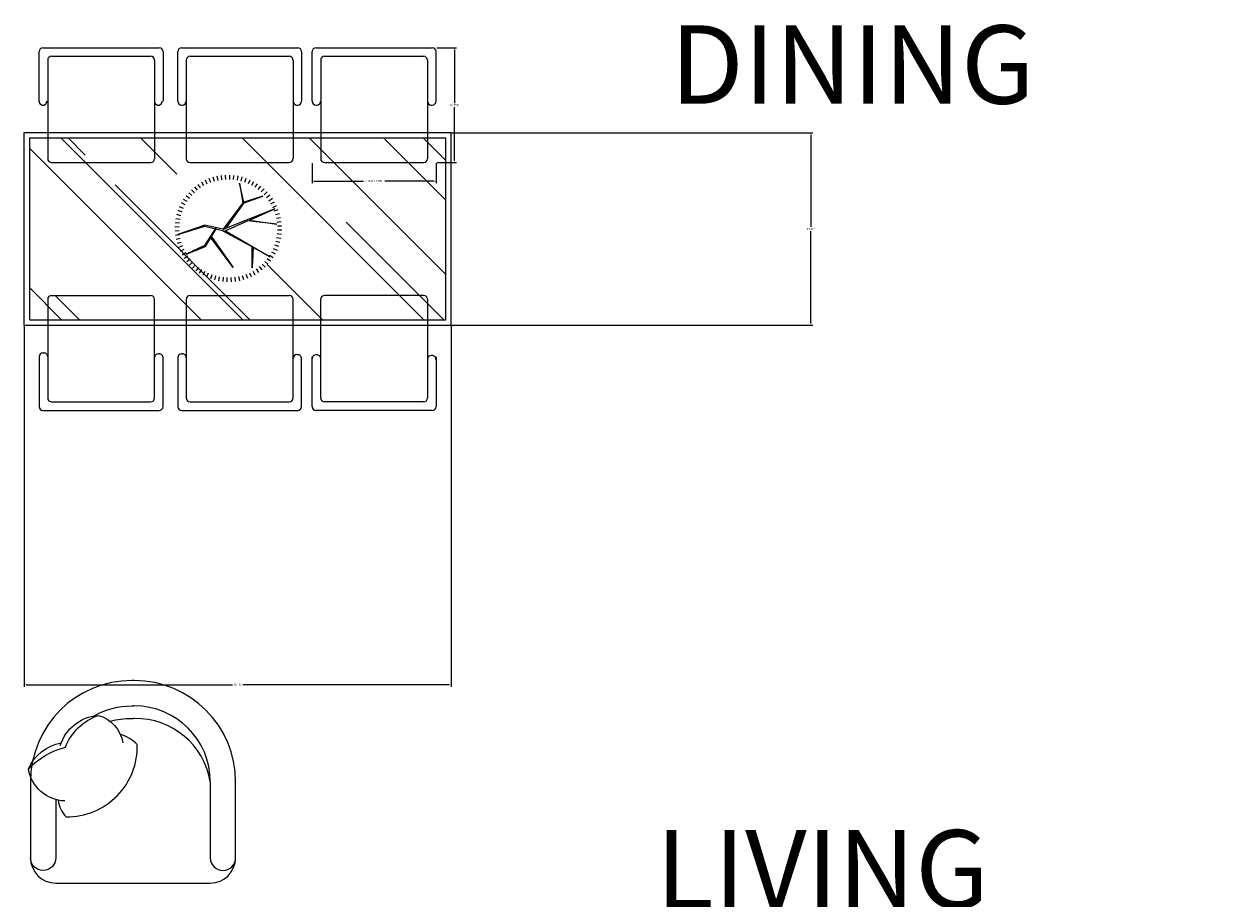
# Model space of a CAD drawing. Units: inches. Extents: x 1676 to 2199, y 1657 to 2783.
# Tile 4 of 10: x 1788 to 1895, y 1985 to 2063. Entities that reach past the tile are written whole.
import ezdxf

# ---------------------------------------------------------------- set-up
doc = ezdxf.new("R2010")
doc.units = ezdxf.units.IN
for name, color, linetype, lineweight in [('A-ANNO-DIMS', 2, 'Continuous', 18), ('A-AREA-IDEN', 7, 'Continuous', 18), ('A-FURN', 8, 'Continuous', 13), ('A-FURN-PATT', 8, 'Continuous', 13)]:
    doc.layers.add(name, color=color, linetype=linetype, lineweight=lineweight)
doc.styles.get("Standard").update_dxf_attribs({"font": 'arial.ttf'})
doc.dimstyles.get("Standard").update_dxf_attribs({"dimtxt": 0.18, "dimasz": 0.18, "dimexe": 0.18, "dimexo": 0.0625, "dimgap": 0.09, "dimtad": 0, "dimtih": 1, "dimtoh": 1, "dimdec": 4, "dimzin": 0, "dimdsep": 46, "dimtxsty": 'Standard', "dimcen": 0.09, "dimadec": 0, "dimazin": 0, "dimtfac": 1, "dimtdec": 4, "dimtofl": 0, "dimtmove": 0, "dimatfit": 3, "dimfxl": 1, "dimtolj": 1, "dimtzin": 0, "dimarcsym": 0})

# ---------------------------------------------------------------- blocks, each defined once
blk = doc.blocks.new('CHAIR-DINING')
for p, q in [((-1.11, 5.48), (-1.11, 9.92)), ((-0.76, 10.27), (9.62, 10.27)), ((9.96, 9.92), (9.96, 5.48)), ((-0.34, 9.16), (-0.34, 0.34)), ((0, 9.5), (8.85, 9.5)), ((9.2, 9.16), (9.2, 0.34)), ((-0.76, 5.13), (-0.69, 5.13)), ((9.54, 5.13), (9.62, 5.13)), ((0, 0), (8.85, 0))]:
    blk.add_line(p, q)
for centre, start, end in [((-0.76, 9.92), 90, 180), ((9.62, 9.92), 0, 90), ((0, 9.16), 90, 180), ((8.85, 9.16), 0, 90), ((-0.76, 5.48), 180, 270), ((-0.69, 5.48), 270, 0), ((9.54, 5.48), 180, 270), ((9.62, 5.48), 270, 0), ((0, 0.34), 180, 270), ((8.85, 0.34), 270, 0)]:
    blk.add_arc(centre, 0.343, start, end)
blk = doc.blocks.new('*D17')
at = {"layer": 'A-ANNO-DIMS', "color": 0, "lineweight": -2, "transparency": 16777216}
for p, q in [((1813.71, 2050.79), (1813.71, 2049.02)), ((1824.78, 2050.79), (1824.78, 2049.02)), ((1813.89, 2049.2), (1818.29, 2049.2)), ((1824.6, 2049.2), (1820.2, 2049.2))]:
    blk.add_line(p, q, dxfattribs=at)
at = {"layer": 'A-ANNO-DIMS', "color": 0, "transparency": 16777216}
for points in [[(1813.89, 2049.23), (1813.89, 2049.17), (1813.71, 2049.2)], [(1824.6, 2049.23), (1824.6, 2049.17), (1824.78, 2049.2)]]:
    blk.add_solid(points, dxfattribs=at)
at = {"layer": 'Defpoints', "color": 0, "transparency": 16777216}
for p in [(1813.71, 2050.86), (1824.78, 2050.86), (1824.78, 2049.2)]:
    blk.add_point(p, dxfattribs=at)
at = {"layer": 'A-ANNO-DIMS', "color": 0, "transparency": 16777216, "insert": (1819.25, 2049.2), "char_height": 0.18, "attachment_point": 5}
blk.add_mtext('\\A1;CHAIR 11 TYP.', dxfattribs=at)
blk = doc.blocks.new('*D18')
at = {"layer": 'A-ANNO-DIMS', "color": 0, "lineweight": -2, "transparency": 16777216}
for p, q in [((1824.84, 2061.12), (1826.62, 2061.12)), ((1826.44, 2060.94), (1826.44, 2056.17)), ((1826.44, 2051.04), (1826.44, 2055.81)), ((1824.84, 2050.86), (1826.62, 2050.86))]:
    blk.add_line(p, q, dxfattribs=at)
at = {"layer": 'A-ANNO-DIMS', "color": 0, "transparency": 16777216}
for points in [[(1826.41, 2060.94), (1826.47, 2060.94), (1826.44, 2061.12)], [(1826.41, 2051.04), (1826.47, 2051.04), (1826.44, 2050.86)]]:
    blk.add_solid(points, dxfattribs=at)
at = {"layer": 'Defpoints', "color": 0, "transparency": 16777216}
for p in [(1824.78, 2061.12), (1826.44, 2061.12), (1824.78, 2050.86)]:
    blk.add_point(p, dxfattribs=at)
at = {"layer": 'A-ANNO-DIMS', "color": 0, "transparency": 16777216, "insert": (1826.44, 2055.99), "char_height": 0.18, "attachment_point": 5}
blk.add_mtext('\\A1;10 TYP.', dxfattribs=at)
blk = doc.blocks.new('*D54')
at = {"layer": 'A-ANNO-DIMS', "color": 0, "lineweight": -2, "transparency": 16777216}
for p, q in [((1787.97, 2036.27), (1787.97, 2004)), ((1826.13, 2036.27), (1826.13, 2004)), ((1788.15, 2004.18), (1806.59, 2004.18)), ((1825.95, 2004.18), (1807.51, 2004.18))]:
    blk.add_line(p, q, dxfattribs=at)
at = {"layer": 'A-ANNO-DIMS', "color": 0, "transparency": 16777216}
for points in [[(1788.15, 2004.21), (1788.15, 2004.15), (1787.97, 2004.18)], [(1825.95, 2004.21), (1825.95, 2004.15), (1826.13, 2004.18)]]:
    blk.add_solid(points, dxfattribs=at)
at = {"layer": 'Defpoints', "color": 0, "transparency": 16777216}
for p in [(1787.97, 2036.33), (1826.13, 2036.33), (1787.97, 2004.18)]:
    blk.add_point(p, dxfattribs=at)
at = {"layer": 'A-ANNO-DIMS', "color": 0, "transparency": 16777216, "insert": (1807.05, 2004.18), "char_height": 0.18, "attachment_point": 5}
blk.add_mtext('\\A1;38.164', dxfattribs=at)
blk = doc.blocks.new('*D55')
at = {"layer": 'A-ANNO-DIMS', "color": 0, "lineweight": -2, "transparency": 16777216}
for p, q in [((1826.2, 2053.5), (1858.46, 2053.5)), ((1858.28, 2053.32), (1858.28, 2045.1)), ((1858.28, 2036.51), (1858.28, 2044.74)), ((1826.2, 2036.33), (1858.46, 2036.33))]:
    blk.add_line(p, q, dxfattribs=at)
at = {"layer": 'A-ANNO-DIMS', "color": 0, "transparency": 16777216}
for points in [[(1858.25, 2053.32), (1858.31, 2053.32), (1858.28, 2053.5)], [(1858.25, 2036.51), (1858.31, 2036.51), (1858.28, 2036.33)]]:
    blk.add_solid(points, dxfattribs=at)
at = {"layer": 'Defpoints', "color": 0, "transparency": 16777216}
for p in [(1826.13, 2053.5), (1826.13, 2036.33), (1858.28, 2036.33)]:
    blk.add_point(p, dxfattribs=at)
at = {"layer": 'A-ANNO-DIMS', "color": 0, "transparency": 16777216, "insert": (1858.28, 2044.92), "char_height": 0.18, "attachment_point": 5}
blk.add_mtext('\\A1;17.174', dxfattribs=at)

msp = doc.modelspace()

# ---------------------------------------------------------------- hatches: boundary and pattern name
at = {"layer": 'A-FURN-PATT'}
h = msp.add_hatch(dxfattribs=at)
h.set_pattern_fill('AR-RROOF', color=256, scale=11.449163, angle=-45, style=0)
h.set_pattern_definition([(315, (2164.764, 3007.215), (25.9065, -9.71494), [171.7375, -22.8983, 57.2458, -11.4492]), (315, (2179.579, 3000.495), (2.6716, 18.86317), [34.3475, -3.7782, 68.695, -8.5869]), (315, (2175.693, 3010.048), (47.522235, -36.67389), [91.5933, -16.02883, 45.79665, -11.44916])])
h.paths.add_polyline_path([(1788.4461, 2036.8061), (1825.6559, 2036.8061), (1825.6559, 2053.0257), (1788.4461, 2053.0257)])

# ---------------------------------------------------------------- linework, layer by layer
at = {"layer": 'A-FURN'}
for p, q in [((1789.3226, 2056.3323), (1789.3226, 2060.7787)), ((1789.666, 2061.1221), (1800.0466, 2061.1221)), ((1800.3901, 2060.7787), (1800.3901, 2056.3323)), ((1790.0858, 2060.0154), (1790.0858, 2051.199)), ((1790.4293, 2060.3589), (1799.2833, 2060.3589)), ((1799.6268, 2060.0154), (1799.6268, 2051.199)), ((1789.666, 2055.9888), (1789.7424, 2055.9888)), ((1799.9703, 2055.9888), (1800.0466, 2055.9888)), ((1826.1329, 2053.5028), (1787.969, 2053.5028)), ((1787.969, 2053.5028), (1787.969, 2036.329)), ((1826.1329, 2036.329), (1826.1329, 2053.5028)), ((1825.6559, 2053.0257), (1788.4461, 2053.0257)), ((1788.4461, 2053.0257), (1788.4461, 2036.8061)), ((1825.6559, 2036.8061), (1825.6559, 2053.0257)), ((1790.4293, 2050.8555), (1799.2833, 2050.8555)), ((1803.743, 2048.5876), (1803.5272, 2048.9023)), ((1804.0346, 2048.7712), (1803.8442, 2049.1019)), ((1804.3398, 2048.9313), (1804.1759, 2049.2759)), ((1804.6566, 2049.067), (1804.5202, 2049.4234)), ((1804.983, 2049.1774), (1804.875, 2049.5434)), ((1805.3171, 2049.2618), (1805.2382, 2049.6352)), ((1805.6568, 2049.3198), (1805.6074, 2049.6983)), ((1806, 2049.351), (1805.9804, 2049.7321)), ((1806.3446, 2049.3551), (1806.355, 2049.7366)), ((1806.6884, 2049.3322), (1806.7287, 2049.7117)), ((1807.0294, 2049.2824), (1807.0994, 2049.6576)), ((1807.2248, 2049.0272), (1807.5315, 2047.2539)), ((1807.5997, 2047.3221), (1807.2248, 2049.0272)), ((1807.3655, 2049.206), (1807.4646, 2049.5745)), ((1807.6945, 2049.1034), (1807.8222, 2049.463)), ((1808.0144, 2048.9754), (1808.17, 2049.3239)), ((1808.3233, 2048.8226), (1808.5058, 2049.1578)), ((1808.6193, 2048.6461), (1808.8275, 2048.9659)), ((1802.7459, 2047.6435), (1802.4434, 2047.8761)), ((1802.9666, 2047.9082), (1802.6832, 2048.1638)), ((1803.2073, 2048.1548), (1802.9449, 2048.4319)), ((1803.4667, 2048.3817), (1803.2268, 2048.6785)), ((1809.3036, 2047.8677), (1807.5997, 2047.3221)), ((1807.6337, 2047.2539), (1809.3036, 2047.8677)), ((1808.9005, 2048.4469), (1809.1331, 2048.7494)), ((1809.1652, 2048.2263), (1809.4209, 2048.5096)), ((1809.4118, 2047.9855), (1809.6889, 2048.2479)), ((1809.6387, 2047.7262), (1809.9356, 2047.966)), ((1802.2175, 2046.7574), (1801.869, 2046.913)), ((1802.3702, 2047.0663), (1802.035, 2047.2488)), ((1802.5467, 2047.3623), (1802.2269, 2047.5705)), ((1807.5315, 2047.2539), (1805.7253, 2044.8668)), ((1810.3941, 2046.7083), (1805.7253, 2044.8668)), ((1805.9639, 2044.9009), (1807.6337, 2047.2539)), ((1808.1204, 2045.7183), (1810.3941, 2046.7083)), ((1809.8446, 2047.4498), (1810.1593, 2047.6657)), ((1810.0282, 2047.1582), (1810.3589, 2047.3487)), ((1810.1883, 2046.853), (1810.5329, 2047.017)), ((1801.9104, 2045.7724), (1801.5353, 2045.8424)), ((1801.9869, 2046.1084), (1801.6183, 2046.2076)), ((1802.0894, 2046.4374), (1801.7298, 2046.5652)), ((1805.9298, 2044.7645), (1807.9425, 2045.6409)), ((1810.5645, 2045.3443), (1807.9425, 2045.6409)), ((1808.1204, 2045.7183), (1810.5645, 2045.3443)), ((1810.324, 2046.5363), (1810.6804, 2046.6726)), ((1810.4344, 2046.2098), (1810.8004, 2046.3178)), ((1810.5189, 2045.8757), (1810.8922, 2045.9547)), ((1801.8377, 2045.0876), (1801.4562, 2045.098)), ((1801.8418, 2044.743), (1801.4607, 2044.7234)), ((1801.8606, 2045.4314), (1801.4811, 2045.4717)), ((1804.1237, 2045.2761), (1801.7041, 2044.4235)), ((1801.7041, 2044.4235), (1804.1237, 2045.1738)), ((1805.1119, 2045.0374), (1804.0896, 2043.4346)), ((1805.7253, 2044.9009), (1804.1237, 2045.2761)), ((1804.1237, 2045.1738), (1805.9298, 2044.7304)), ((1804.1918, 2043.3664), (1805.146, 2044.935)), ((1808.3494, 2043.3187), (1805.7594, 2044.7304)), ((1805.9639, 2044.7645), (1809.9511, 2042.4457)), ((1810.5768, 2045.536), (1810.9553, 2045.5854)), ((1810.608, 2045.1928), (1810.9891, 2045.2124)), ((1810.6121, 2044.8482), (1810.9936, 2044.8378)), ((1801.873, 2044.3998), (1801.4946, 2044.3504)), ((1801.931, 2044.0601), (1801.5576, 2043.9812)), ((1802.0155, 2043.726), (1801.6494, 2043.618)), ((1806.6455, 2041.4908), (1804.6348, 2044.1848)), ((1804.7371, 2044.1848), (1806.6455, 2041.4908)), ((1810.3604, 2043.4984), (1810.72, 2043.3706)), ((1810.463, 2043.8274), (1810.8315, 2043.7282)), ((1810.5394, 2044.1634), (1810.9146, 2044.0935)), ((1810.5892, 2044.5044), (1810.9687, 2044.4641)), ((1802.1259, 2043.3996), (1801.7694, 2043.2632)), ((1802.2616, 2043.0828), (1801.9169, 2042.9189)), ((1802.4217, 2042.7776), (1802.091, 2042.5872)), ((1802.6053, 2042.486), (1802.2905, 2042.2702)), ((1804.0896, 2043.4346), (1802.4538, 2042.6844)), ((1802.4538, 2042.6844), (1804.1918, 2043.3664)), ((1808.3494, 2041.4567), (1808.3494, 2043.3187)), ((1808.4295, 2043.275), (1808.3494, 2041.4567)), ((1809.9511, 2042.4457), (1808.4295, 2043.275)), ((1809.9031, 2042.5736), (1810.223, 2042.3654)), ((1810.0796, 2042.8695), (1810.4148, 2042.6871)), ((1810.2324, 2043.1784), (1810.5809, 2043.0228)), ((1802.8111, 2042.2096), (1802.5143, 2041.9698)), ((1803.0381, 2041.9503), (1802.761, 2041.6879)), ((1803.2847, 2041.7096), (1803.029, 2041.4262)), ((1803.5494, 2041.4889), (1803.3167, 2041.1864)), ((1808.7069, 2041.3482), (1808.9227, 2041.0335)), ((1808.9832, 2041.5541), (1809.223, 2041.2573)), ((1809.2425, 2041.7811), (1809.5049, 2041.5039)), ((1809.4833, 2042.0276), (1809.7666, 2041.772)), ((1809.7039, 2042.2924), (1810.0064, 2042.0597)), ((1803.8306, 2041.2897), (1803.6224, 2040.9699)), ((1804.1265, 2041.1132), (1803.9441, 2040.778)), ((1804.4355, 2040.9604), (1804.2798, 2040.612)), ((1804.7554, 2040.8324), (1804.6276, 2040.4728)), ((1805.0844, 2040.7299), (1804.9852, 2040.3613)), ((1805.4204, 2040.6534), (1805.3505, 2040.2783)), ((1805.7614, 2040.6036), (1805.7211, 2040.2241)), ((1806.1053, 2040.5807), (1806.0949, 2040.1992)), ((1806.4498, 2040.5848), (1806.4694, 2040.2037)), ((1806.793, 2040.616), (1806.8424, 2040.2376)), ((1807.1327, 2040.674), (1807.2117, 2040.3006)), ((1807.4668, 2040.7584), (1807.5748, 2040.3924)), ((1807.7933, 2040.8689), (1807.9297, 2040.5124)), ((1808.1101, 2041.0045), (1808.274, 2040.6599)), ((1808.4152, 2041.1647), (1808.6057, 2040.834)), ((1790.0858, 2038.6328), (1790.0858, 2029.8164)), ((1790.4293, 2038.9762), (1799.2833, 2038.9762)), ((1799.6268, 2029.8164), (1799.6268, 2038.6328)), ((1802.465, 2038.6328), (1802.465, 2029.8164)), ((1802.8084, 2038.9762), (1811.6625, 2038.9762)), ((1812.0059, 2029.8164), (1812.0059, 2038.6328)), ((1814.4751, 2029.8164), (1814.4751, 2038.6328)), ((1823.6726, 2038.9762), (1814.8186, 2038.9762)), ((1824.0161, 2038.6328), (1824.0161, 2029.8164)), ((1787.969, 2036.329), (1826.1329, 2036.329)), ((1788.4461, 2036.8061), (1825.6559, 2036.8061)), ((1789.6683, 2033.8406), (1789.7446, 2033.8401)), ((1789.3226, 2033.4995), (1789.3226, 2029.0531)), ((1799.9723, 2033.7724), (1800.0487, 2033.7718)), ((1800.3901, 2029.0531), (1800.3901, 2033.4995)), ((1801.7017, 2033.4995), (1801.7017, 2029.0531)), ((1802.0472, 2033.7586), (1802.1235, 2033.7581)), ((1812.3512, 2033.6903), (1812.4275, 2033.6898)), ((1812.7692, 2029.0531), (1812.7692, 2033.4995)), ((1813.7118, 2029.0531), (1813.7118, 2033.4995)), ((1814.1334, 2033.6785), (1814.057, 2033.679)), ((1824.4374, 2033.6102), (1824.3611, 2033.6107)), ((1824.7794, 2033.4995), (1824.7794, 2029.0531)), ((1789.666, 2028.7096), (1800.0466, 2028.7096)), ((1790.4293, 2029.4729), (1799.2833, 2029.4729)), ((1802.0452, 2028.7096), (1812.4257, 2028.7096)), ((1802.8084, 2029.4729), (1811.6625, 2029.4729)), ((1824.4359, 2028.7096), (1814.0553, 2028.7096)), ((1823.6726, 2029.4729), (1814.8186, 2029.4729))]:
    msp.add_line(p, q, dxfattribs=at)
at = {"layer": 'A-FURN', "ltscale": 0.03}
msp.add_lwpolyline([(1797.7122, 1986.4536), (1804.6154, 1986.4536, 0.41421356), (1806.8787, 1988.7169), (1806.8787, 1995.5069, 0.41421356), (1797.8254, 2004.5603), (1797.7122, 2004.5603), (1797.5991, 2004.5603, 0.41421356), (1788.5457, 1995.5069), (1788.5457, 1988.7169, 0.41421356), (1790.8091, 1986.4536), (1797.7122, 1986.4536)], format="xyb", dxfattribs=at)
at = {"layer": 'A-FURN'}
for points in [[(1794.2286, 2001.4014, -0.13059149), (1797.5991, 2002.2969), (1797.7122, 2002.2969)], [(1804.6154, 1995.5069, 0.41421356), (1797.8254, 2002.2969), (1797.7122, 2002.2969)], [(1788.3606, 1996.6493, -0.14772988), (1791.6682, 1998.5942, -0.21334276), (1794.5866, 2001.4467, -0.17866181)], [(1791.2112, 1998.7492, -0.30666349), (1794.5866, 2001.4467, -0.30632997), (1796.7916, 1998.9832, 0.87284716)], [(1795.6696, 2000.9214, -0.07238424), (1797.5991, 2001.1653), (1797.7122, 2001.1653)], [(1804.6154, 1995.5069, 0.37271891), (1797.8254, 2001.1653), (1797.7122, 2001.1653)], [(1791.0329, 1993.8658, 0.16554063), (1791.733, 1992.3706, 0.42598917), (1798.0887, 1998.8535, 0.12152332), (1796.58, 1999.7471, -7.11546429)], [(1791.6033, 1993.7968, -0.35677236), (1788.3606, 1996.6493, -0.24954205), (1791.2988, 1999, 9.61688035)], [(1804.6154, 1995.5071), (1804.6154, 1988.7169, 0.41421356), (1805.7471, 1987.5853), (1805.7471, 1987.5853, 0.41421356), (1806.8787, 1988.7169)], [(1790.8091, 1993.9202), (1790.8091, 1988.7169, -0.41421356), (1789.6774, 1987.5853), (1789.6774, 1987.5853, -0.41421356), (1788.5457, 1988.7169)]]:
    msp.add_lwpolyline(points, format="xyb", dxfattribs=at)
for centre, start, end in [((1789.666, 2060.7787), 90, 180), ((1800.0466, 2060.7787), 0, 90), ((1790.4293, 2060.0154), 90, 180), ((1799.2833, 2060.0154), 0, 90), ((1789.666, 2056.3323), 180, 0.103974), ((1799.9703, 2056.3323), 180, 0.103974), ((1790.4293, 2051.199), 180, 270), ((1799.2833, 2051.199), 270, 0), ((1790.4293, 2038.6328), 90, 180), ((1799.2833, 2038.6328), 0, 90), ((1802.8084, 2038.6328), 90, 180), ((1811.6625, 2038.6328), 0, 90), ((1814.8186, 2038.6328), 90, 180), ((1823.6726, 2038.6328), 0, 90), ((1789.666, 2033.4972), 89.620247, 179.620246), ((1789.7424, 2033.4967), 359.620246, 89.620247), ((1799.9701, 2033.4289), 89.620247, 179.620246), ((1800.0464, 2033.4284), 359.620246, 89.620247), ((1802.0449, 2033.4151), 89.620247, 179.620246), ((1802.1212, 2033.4146), 359.620246, 89.620247), ((1812.3489, 2033.3468), 89.620247, 179.620246), ((1812.4252, 2033.3463), 359.620246, 89.620247), ((1814.0548, 2033.3355), 89.620247, 179.620246), ((1814.1311, 2033.335), 359.620246, 89.620247), ((1824.3588, 2033.2672), 89.620247, 179.620246), ((1824.4351, 2033.2667), 359.620246, 89.620247), ((1790.4293, 2029.8164), 180, 270), ((1799.2833, 2029.8164), 270, 0), ((1802.8084, 2029.8164), 180, 270), ((1811.6625, 2029.8164), 270, 0), ((1814.8186, 2029.8164), 180, 270), ((1823.6726, 2029.8164), 270, 0), ((1789.666, 2029.0531), 180, 270), ((1800.0466, 2029.0531), 270, 0), ((1802.0452, 2029.0531), 180, 270), ((1812.4257, 2029.0531), 270, 0), ((1814.0553, 2029.0531), 180, 270), ((1824.4359, 2029.0531), 270, 0)]:
    msp.add_arc(centre, 0.3435, start, end, dxfattribs=at)

# ---------------------------------------------------------------- block references
for p in [(1802.8084, 2050.8555), (1814.8186, 2050.8555)]:
    msp.add_blockref('CHAIR-DINING', p, dxfattribs=at)

# ---------------------------------------------------------------- texts
at = {"layer": 'A-AREA-IDEN', "char_height": 7, "attachment_point": 1}
for s, width, insert in [('DINING', 69.533341, (1845.7127, 2063.1188)), ('LIVING \\P14\'7"X16\'1"', 86.067539, (1844.4148, 1991.1927))]:
    msp.add_mtext_dynamic_manual_height_columns(s, width=width, gutter_width=12.5, heights=[0], dxfattribs=dict(at, insert=insert))

# ---------------------------------------------------------------- dimensions: what is measured, and where the dimension line sits
at = {"layer": 'A-ANNO-DIMS'}
dim = msp.add_linear_dim(base=(1826.4395, 2061.1221), p1=(1824.7794, 2050.8555), p2=(1824.7794, 2061.1221), angle=90, text='<> TYP.', dimstyle='Standard', override={"dimdec": 0, "dimlfac": 1, "dimrnd": 0, "dimzin": 0, "dimdsep": 46, "dimlunit": 2}, dxfattribs=at)
dim.commit()
dim.dimension.update_dxf_attribs({"geometry": '*D18', "text_midpoint": (1826.4395, 2055.9888)})
for base, p1, p2, angle, picture, middle in [((1858.2829, 2036.329), (1826.1329, 2053.5028), (1826.1329, 2036.329), 270, '*D55', (1858.2829, 2044.9159)), ((1787.969, 2004.179), (1826.1329, 2036.329), (1787.969, 2036.329), 180, '*D54', (1807.051, 2004.179))]:
    dim = msp.add_linear_dim(base=base, p1=p1, p2=p2, angle=angle, dimstyle='Standard', override={"dimdec": 3, "dimlfac": 1, "dimrnd": 0, "dimzin": 0, "dimdsep": 46, "dimlunit": 2}, dxfattribs=at)
    dim.commit()
    dim.dimension.update_dxf_attribs({"geometry": picture, "text_midpoint": middle})
dim = msp.add_linear_dim(base=(1824.7794, 2049.1954), p1=(1813.7118, 2050.8555), p2=(1824.7794, 2050.8555), text='CHAIR <> TYP.', dimstyle='Standard', override={"dimdec": 0, "dimlfac": 1, "dimrnd": 0, "dimzin": 0, "dimdsep": 46, "dimlunit": 2}, dxfattribs=at)
dim.commit()
dim.dimension.update_dxf_attribs({"geometry": '*D17', "text_midpoint": (1819.2456, 2049.1954)})

doc.saveas('drawing.dxf')
